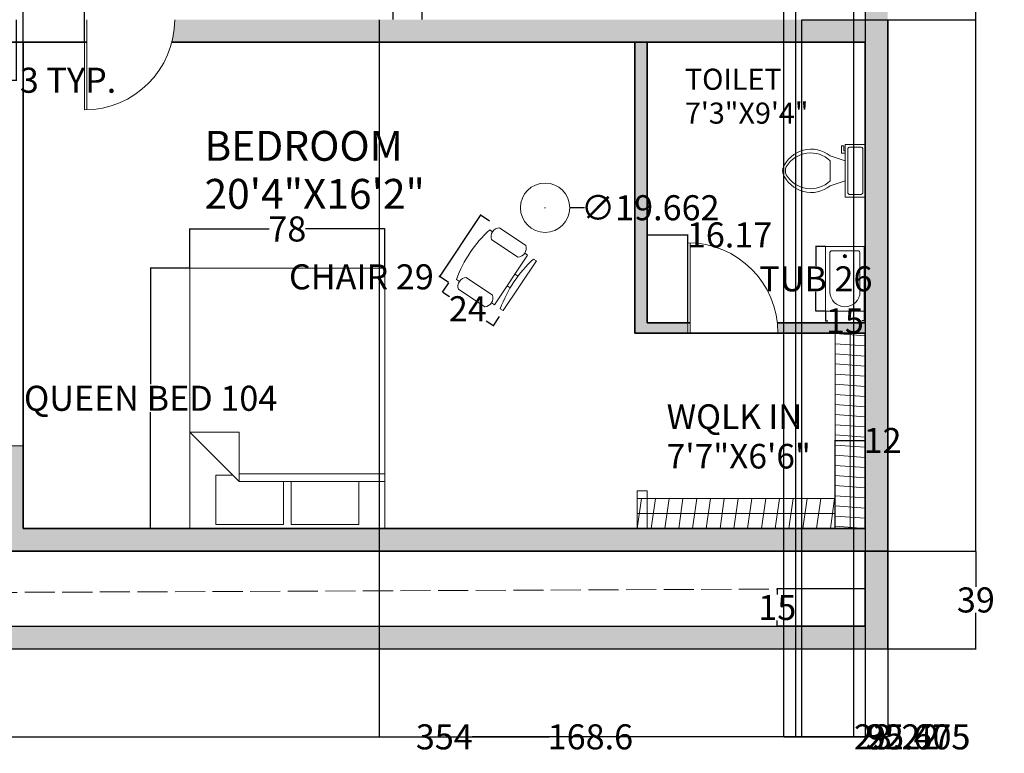
# Model space of a CAD drawing. Units: inches. Extents: x 409 to 1056, y 160 to 945.
# Tile 2 of 6: x 625 to 1018, y 160 to 453. Entities that reach past the tile are written whole.
import ezdxf

# ---------------------------------------------------------------- set-up
doc = ezdxf.new("R2010")
doc.units = ezdxf.units.IN
doc.header["$MEASUREMENT"] = 0
doc.linetypes.add('ACAD_ISO02W100', pattern=[15, 12, -3])
for name, color, linetype, lineweight in [('A-ANNO-DIMS', 2, 'Continuous', 18), ('A-AREA-IDEN', 7, 'Continuous', 18), ('A-DOOR', 3, 'Continuous', 18), ('A-FLOR-CASE', 8, 'Continuous', 20), ('A-FLOR-CASE-PATT', 9, 'Continuous', 13), ('A-FLOR-FIXT', 8, 'Continuous', 18), ('A-FURN', 8, 'Continuous', 18), ('A-GLAZ', 4, 'Continuous', 18), ('A-ROOF-BYND', 8, 'ACAD_ISO02W100', 13), ('A-WALL', 7, 'Continuous', 35), ('A-WALL-PRPT', 7, 'Continuous', 30)]:
    doc.layers.add(name, color=color, linetype=linetype, lineweight=lineweight)
doc.layers.add('A-WALL-PATT', color=251, linetype='Continuous', lineweight=13, true_color=0x636466)
doc.styles.get("Standard").update_dxf_attribs({"font": 'arial.ttf'})
doc.dimstyles.get("Standard").update_dxf_attribs({"dimtxt": 10, "dimasz": 0.18, "dimexe": 0.18, "dimexo": 0.0625, "dimgap": 0.09, "dimtad": 0, "dimtih": 1, "dimtoh": 1, "dimdec": 0, "dimzin": 0, "dimdsep": 46, "dimlunit": 3, "dimtxsty": 'Standard', "dimcen": 0.09, "dimadec": 0, "dimazin": 0, "dimtfac": 1, "dimtdec": 0, "dimtofl": 0, "dimtmove": 0, "dimatfit": 3, "dimfxl": 1, "dimtolj": 1, "dimtzin": 0, "dimarcsym": 0})

# ---------------------------------------------------------------- blocks, each defined once
blk = doc.blocks.new('Bath Tub - 26 x 60 in.')
for p, q in [((8, -18), (10, -18)), ((9, -17), (9, -19))]:
    blk.add_line(p, q)
blk.add_lwpolyline([(0, -36), (0, 0), (60, 0), (60, -36)], close=True)
for points in [[(4, -30), (4, -6)], [(6, -4), (42, -4)], [(42, -32), (6, -32)]]:
    blk.add_lwpolyline(points)
for radius in [1.5, 1]:
    blk.add_circle((9, -18), radius)
for centre, radius, start, end in [((5.75, -5.75), 1.77, 81.8699, 188.1301), ((42, -18), 14, 270, 90), ((5.75, -30.25), 1.77, 171.8699, 278.1301)]:
    blk.add_arc(centre, radius, start, end)
blk = doc.blocks.new('Toilet - top')
for p, q in [((9.5, -6), (9.5, -2)), ((-10, -8.5), (-8, -8.5)), ((-10, -9.5), (-10, -8.5)), ((-7, -9.5), (-10, -9.5)), ((-8, -8.5), (-8, -8)), ((-7, -8), (-7, -9.5)), ((-4, -8), (-6, -14)), ((4, -8), (6, -14)), ((4, -14), (-4, -14))]:
    blk.add_line(p, q)
blk.add_lwpolyline([(10.5, -8), (10.5, 0), (-10.5, 0), (-10.5, -8)], close=True)
for points in [[(-9.5, -2), (-9.5, -6)], [(8.5, -1), (-8.5, -1)], [(-8.5, -7), (8.5, -7)]]:
    blk.add_lwpolyline(points)
for centre, radius, start, end in [((-8.62, -1.88), 0.884, 81.8699, 188.1301), ((8.62, -1.88), 0.884, 351.8699, 98.1301), ((-8.62, -6.12), 0.884, 171.8699, 278.1301), ((8.62, -6.12), 0.884, 261.8699, 8.1301), ((3.52, -21.58), 12.17, 141.4691, 247.9714), ((4.2, -21.82), 11.33, 136.3677, 238.9468), ((-3.52, -21.58), 12.17, 292.0284, 38.5307), ((-4.2, -21.82), 11.33, 301.053, 43.6321), ((0, -27.88), 4, 245.7318, 294.2682), ((0, -29), 4, 254.8605, 285.1395)]:
    blk.add_arc(centre, radius, start, end)
blk = doc.blocks.new('Bed - Queen')
for p, q in [((0, -80.00003), (0, 0)), ((0, 0), (59.99999, 0)), ((59.99999, 0), (59.99999, -80.00003)), ((7.99999, -1.2), (28.79998, -1.2)), ((7.99999, -14.4), (7.99999, -1.2)), ((28.79998, -1.2), (28.79998, -14.4)), ((31.19999, -1.2), (51.99999, -1.2)), ((31.19999, -14.4), (31.19999, -1.2)), ((51.99999, -1.2), (51.99999, -16.4)), ((0, -14.4), (44.8, -14.4)), ((59.99999, -29.6), (44.8, -14.4)), ((44.8, -14.4), (44.8, -29.6)), ((44.8, -16.8), (0, -16.8)), ((51.99999, -16.4), (46.79936, -16.4)), ((44.8, -29.6), (59.99999, -29.6)), ((59.99999, -80.00003), (0, -80.00003))]:
    blk.add_line(p, q)
blk = doc.blocks.new('Chair - Desk')
for p, q in [((-8.5, 0), (-8.5, -1)), ((-8.5, 0), (8.5, 0)), ((8.5, 0), (8.5, -1)), ((-2, -3), (-2, -1.9355)), ((2, -1.9576), (2, -3)), ((-10.5, -5), (-10.5, -14)), ((-8.5, -3), (-8.5, -4)), ((-8.5, -3), (8.5, -3)), ((-6.5, -14), (-6.5, -5)), ((6.5, -5), (6.5, -14)), ((8.5, -3), (8.5, -4)), ((10.5, -14), (10.5, -5)), ((-8.5, -15), (-8.5, -16)), ((8.5, -15), (8.5, -16))]:
    blk.add_line(p, q)
for centre, radius, start, end in [((0, 34.625), 36.625, 256.5803, 283.4197), ((-8.5, -6.5), 2.5, 36.8699, 143.1301), ((8.5, -6.5), 2.5, 36.8699, 143.1301), ((-8.5, -12.5), 2.5, 216.8699, 323.1301), ((8.5, -12.5), 2.5, 216.8699, 323.1301), ((0, 19.625), 36.625, 256.5803, 283.4197)]:
    blk.add_arc(centre, radius, start, end)
blk = doc.blocks.new('DOOR-SWING-36IN')
for p, q in [((35, 36), (35, 0)), ((36, 36), (36, 0))]:
    blk.add_line(p, q)
blk.add_arc((36, 36), 36, 180, 270)
blk = doc.blocks.new('*D14')
at = {"layer": 'A-ANNO-DIMS', "color": 0, "lineweight": -2, "transparency": 16777216}
for p, q in [((620.85, 452.68), (620.85, 428.41)), ((623.85, 452.68), (623.85, 428.41)), ((621.03, 428.59), (623.67, 428.59)), ((623.85, 428.59), (624.03, 428.59))]:
    blk.add_line(p, q, dxfattribs=at)
at = {"layer": 'A-ANNO-DIMS', "color": 0, "transparency": 16777216}
for points in [[(621.03, 428.62), (621.03, 428.56), (620.85, 428.59)], [(623.67, 428.62), (623.67, 428.56), (623.85, 428.59)]]:
    blk.add_solid(points, dxfattribs=at)
at = {"layer": 'Defpoints', "color": 0, "transparency": 16777216}
for p in [(620.85, 452.74), (623.85, 452.74), (623.85, 428.59)]:
    blk.add_point(p, dxfattribs=at)
at = {"layer": 'A-ANNO-DIMS', "color": 0, "transparency": 16777216, "insert": (644.57, 428.59), "char_height": 10, "attachment_point": 5}
blk.add_mtext('\\A1;3 TYP.', dxfattribs=at)
blk = doc.blocks.new('*D15')
at = {"layer": 'A-ANNO-DIMS', "color": 0, "lineweight": -2, "transparency": 16777216}
for p, q in [((693.07, 353.66), (677.36, 353.66)), ((677.54, 353.48), (677.54, 307.27)), ((677.54, 249.92), (677.54, 296.13)), ((693.07, 249.74), (677.36, 249.74))]:
    blk.add_line(p, q, dxfattribs=at)
at = {"layer": 'A-ANNO-DIMS', "color": 0, "transparency": 16777216}
for points in [[(677.51, 353.48), (677.57, 353.48), (677.54, 353.66)], [(677.51, 249.92), (677.57, 249.92), (677.54, 249.74)]]:
    blk.add_solid(points, dxfattribs=at)
at = {"layer": 'Defpoints', "color": 0, "transparency": 16777216}
for p in [(693.13, 353.66), (677.54, 249.74), (693.13, 249.74)]:
    blk.add_point(p, dxfattribs=at)
at = {"layer": 'A-ANNO-DIMS', "color": 0, "transparency": 16777216, "insert": (677.54, 301.7), "char_height": 10, "attachment_point": 5}
blk.add_mtext('\\A1;QUEEN BED 104', dxfattribs=at)
blk = doc.blocks.new('*D16')
at = {"layer": 'A-ANNO-DIMS', "color": 0, "lineweight": -2, "transparency": 16777216}
for p, q in [((693.13, 353.72), (693.13, 369.43)), ((771.07, 353.72), (771.07, 369.43)), ((693.31, 369.25), (724.88, 369.25)), ((770.89, 369.25), (739.32, 369.25))]:
    blk.add_line(p, q, dxfattribs=at)
at = {"layer": 'A-ANNO-DIMS', "color": 0, "transparency": 16777216}
for points in [[(693.31, 369.28), (693.31, 369.22), (693.13, 369.25)], [(770.89, 369.28), (770.89, 369.22), (771.07, 369.25)]]:
    blk.add_solid(points, dxfattribs=at)
at = {"layer": 'Defpoints', "color": 0, "transparency": 16777216}
for p in [(693.13, 369.25), (693.13, 353.66), (771.07, 353.66)]:
    blk.add_point(p, dxfattribs=at)
at = {"layer": 'A-ANNO-DIMS', "color": 0, "transparency": 16777216, "insert": (732.1, 369.25), "char_height": 10, "attachment_point": 5}
blk.add_mtext('\\A1;78', dxfattribs=at)
blk = doc.blocks.new('*D17')
at = {"layer": 'A-ANNO-DIMS', "color": 0, "lineweight": -2, "transparency": 16777216}
for p, q in [((809.08, 374.62), (792.92, 350.44)), ((812.8, 372.35), (809.03, 374.87)), ((792.72, 350.15), (792.54, 350.15)), ((796.44, 347.88), (792.67, 350.4)), ((792.82, 350.3), (792.72, 350.15))]:
    blk.add_line(p, q, dxfattribs=at)
at = {"layer": 'A-ANNO-DIMS', "color": 0, "transparency": 16777216}
for points in [[(809.06, 374.64), (809.11, 374.6), (809.18, 374.77)], [(792.9, 350.46), (792.95, 350.43), (792.82, 350.3)]]:
    blk.add_solid(points, dxfattribs=at)
at = {"layer": 'Defpoints', "color": 0, "transparency": 16777216}
for p in [(812.86, 372.31), (792.82, 350.3), (796.49, 347.84)]:
    blk.add_point(p, dxfattribs=at)
at = {"layer": 'A-ANNO-DIMS', "color": 0, "transparency": 16777216, "insert": (761.66, 350.15), "char_height": 10, "attachment_point": 5}
blk.add_mtext('\\A1;CHAIR 29', dxfattribs=at)
blk = doc.blocks.new('*D18')
at = {"layer": 'A-ANNO-DIMS', "color": 0, "lineweight": -2, "transparency": 16777216}
for p, q in [((796.46, 347.79), (793.94, 344.02)), ((794.19, 344.07), (796.82, 342.31)), ((816.66, 334.28), (814.14, 330.51)), ((814.09, 330.76), (811.45, 332.52))]:
    blk.add_line(p, q, dxfattribs=at)
at = {"layer": 'A-ANNO-DIMS', "color": 0, "transparency": 16777216}
for points in [[(794.2, 344.09), (794.17, 344.04), (794.04, 344.17)], [(814.1, 330.79), (814.07, 330.74), (814.24, 330.66)]]:
    blk.add_solid(points, dxfattribs=at)
at = {"layer": 'Defpoints', "color": 0, "transparency": 16777216}
for p in [(796.49, 347.84), (816.69, 334.33), (814.24, 330.66)]:
    blk.add_point(p, dxfattribs=at)
at = {"layer": 'A-ANNO-DIMS', "color": 0, "transparency": 16777216, "insert": (804.14, 337.42), "char_height": 10, "attachment_point": 5}
blk.add_mtext('\\A1;24', dxfattribs=at)
blk = doc.blocks.new('*D29')
at = {"layer": 'A-ANNO-DIMS', "color": 0, "lineweight": -2, "transparency": 16777216}
for p, q in [((946.82, 362.24), (942.84, 362.24)), ((943.02, 362.06), (943.02, 354.55)), ((943.02, 336.65), (943.02, 344.16)), ((946.82, 336.47), (942.84, 336.47))]:
    blk.add_line(p, q, dxfattribs=at)
at = {"layer": 'A-ANNO-DIMS', "color": 0, "transparency": 16777216}
for points in [[(942.99, 362.06), (943.05, 362.06), (943.02, 362.24)], [(942.99, 336.65), (943.05, 336.65), (943.02, 336.47)]]:
    blk.add_solid(points, dxfattribs=at)
at = {"layer": 'Defpoints', "color": 0, "transparency": 16777216}
for p in [(946.88, 362.24), (943.02, 336.47), (946.88, 336.47)]:
    blk.add_point(p, dxfattribs=at)
at = {"layer": 'A-ANNO-DIMS', "color": 0, "transparency": 16777216, "insert": (943.02, 349.36), "char_height": 10, "attachment_point": 5}
blk.add_mtext('\\A1;TUB 26', dxfattribs=at)
blk = doc.blocks.new('*D30')
at = {"layer": 'A-ANNO-DIMS', "color": 0, "lineweight": -2, "transparency": 16777216}
for p, q in [((946.88, 336.41), (946.88, 332.43)), ((962.34, 336.41), (962.34, 332.43)), ((947.06, 332.61), (947.79, 332.61)), ((962.16, 332.61), (961.43, 332.61))]:
    blk.add_line(p, q, dxfattribs=at)
at = {"layer": 'A-ANNO-DIMS', "color": 0, "transparency": 16777216}
for points in [[(947.06, 332.64), (947.06, 332.58), (946.88, 332.61)], [(962.16, 332.64), (962.16, 332.58), (962.34, 332.61)]]:
    blk.add_solid(points, dxfattribs=at)
at = {"layer": 'Defpoints', "color": 0, "transparency": 16777216}
for p in [(946.88, 336.47), (962.34, 336.47), (962.34, 332.61)]:
    blk.add_point(p, dxfattribs=at)
at = {"layer": 'A-ANNO-DIMS', "color": 0, "transparency": 16777216, "insert": (954.61, 332.61), "char_height": 10, "attachment_point": 5}
blk.add_mtext('\\A1;15', dxfattribs=at)
blk = doc.blocks.new('*D37')
at = {"layer": 'A-ANNO-DIMS', "color": 0, "lineweight": -2, "transparency": 16777216}
for p, q in [((617.74, 240.68), (617.74, 166.44)), ((971.74, 240.68), (971.74, 166.44)), ((617.92, 166.62), (783.63, 166.62)), ((971.56, 166.62), (805.85, 166.62))]:
    blk.add_line(p, q, dxfattribs=at)
at = {"layer": 'A-ANNO-DIMS', "color": 0, "transparency": 16777216}
for points in [[(617.92, 166.65), (617.92, 166.59), (617.74, 166.62)], [(971.56, 166.65), (971.56, 166.59), (971.74, 166.62)]]:
    blk.add_solid(points, dxfattribs=at)
at = {"layer": 'Defpoints', "color": 0, "transparency": 16777216}
for p in [(617.74, 240.74), (971.74, 240.74), (971.74, 166.62)]:
    blk.add_point(p, dxfattribs=at)
at = {"layer": 'A-ANNO-DIMS', "color": 0, "transparency": 16777216, "insert": (794.74, 166.62), "char_height": 10, "attachment_point": 5}
blk.add_mtext('\\A1;354', dxfattribs=at)
blk = doc.blocks.new('*D38')
at = {"layer": 'A-ANNO-DIMS', "color": 0, "lineweight": -2, "transparency": 16777216}
for p, q in [((971.8, 810.74), (1007.05, 810.74)), ((1006.87, 810.56), (1006.87, 530.94)), ((1006.87, 240.92), (1006.87, 520.55)), ((971.8, 240.74), (1007.05, 240.74))]:
    blk.add_line(p, q, dxfattribs=at)
at = {"layer": 'A-ANNO-DIMS', "color": 0, "transparency": 16777216}
for points in [[(1006.84, 810.56), (1006.9, 810.56), (1006.87, 810.74)], [(1006.84, 240.92), (1006.9, 240.92), (1006.87, 240.74)]]:
    blk.add_solid(points, dxfattribs=at)
at = {"layer": 'Defpoints', "color": 0, "transparency": 16777216}
for p in [(971.74, 810.74), (1006.87, 810.74), (971.74, 240.74)]:
    blk.add_point(p, dxfattribs=at)
at = {"layer": 'A-ANNO-DIMS', "color": 0, "transparency": 16777216, "insert": (1006.87, 525.74), "char_height": 10, "attachment_point": 5}
blk.add_mtext('\\A1;570', dxfattribs=at)
blk = doc.blocks.new('*D39')
at = {"layer": 'A-ANNO-DIMS', "color": 0, "lineweight": -2, "transparency": 16777216}
for p, q in [((971.8, 240.74), (1007.05, 240.74)), ((1006.87, 240.56), (1006.87, 226.44)), ((1006.87, 201.92), (1006.87, 216.04)), ((971.8, 201.74), (1007.05, 201.74))]:
    blk.add_line(p, q, dxfattribs=at)
at = {"layer": 'A-ANNO-DIMS', "color": 0, "transparency": 16777216}
for points in [[(1006.84, 240.56), (1006.9, 240.56), (1006.87, 240.74)], [(1006.84, 201.92), (1006.9, 201.92), (1006.87, 201.74)]]:
    blk.add_solid(points, dxfattribs=at)
at = {"layer": 'Defpoints', "color": 0, "transparency": 16777216}
for p in [(971.74, 240.74), (1006.87, 240.74), (971.74, 201.74)]:
    blk.add_point(p, dxfattribs=at)
at = {"layer": 'A-ANNO-DIMS', "color": 0, "transparency": 16777216, "insert": (1006.87, 221.24), "char_height": 10, "attachment_point": 5}
blk.add_mtext('\\A1;39', dxfattribs=at)
blk = doc.blocks.new('*D40')
at = {"layer": 'A-ANNO-DIMS', "color": 0, "lineweight": -2, "transparency": 16777216}
for p, q in [((930.07, 622.68), (930.07, 166.44)), ((962.74, 622.68), (962.74, 166.44)), ((930.25, 166.62), (962.56, 166.62)), ((962.74, 166.62), (962.92, 166.62))]:
    blk.add_line(p, q, dxfattribs=at)
at = {"layer": 'A-ANNO-DIMS', "color": 0, "transparency": 16777216}
for points in [[(930.25, 166.65), (930.25, 166.59), (930.07, 166.62)], [(962.56, 166.65), (962.56, 166.59), (962.74, 166.62)]]:
    blk.add_solid(points, dxfattribs=at)
at = {"layer": 'Defpoints', "color": 0, "transparency": 16777216}
for p in [(930.07, 622.74), (962.74, 622.74), (962.74, 166.62)]:
    blk.add_point(p, dxfattribs=at)
at = {"layer": 'A-ANNO-DIMS', "color": 0, "transparency": 16777216, "insert": (983.8, 166.62), "char_height": 10, "attachment_point": 5}
blk.add_mtext('\\A1;32.675', dxfattribs=at)
blk = doc.blocks.new('*D41')
at = {"layer": 'A-ANNO-DIMS', "color": 0, "lineweight": -2, "transparency": 16777216}
for p, q in [((934.87, 626.08), (934.87, 166.44)), ((958.09, 626.08), (958.09, 166.44)), ((935.05, 166.62), (957.91, 166.62)), ((958.09, 166.62), (958.27, 166.62))]:
    blk.add_line(p, q, dxfattribs=at)
at = {"layer": 'A-ANNO-DIMS', "color": 0, "transparency": 16777216}
for points in [[(935.05, 166.65), (935.05, 166.59), (934.87, 166.62)], [(957.91, 166.65), (957.91, 166.59), (958.09, 166.62)]]:
    blk.add_solid(points, dxfattribs=at)
at = {"layer": 'Defpoints', "color": 0, "transparency": 16777216}
for p in [(934.87, 626.14), (958.09, 626.14), (958.09, 166.62)]:
    blk.add_point(p, dxfattribs=at)
at = {"layer": 'A-ANNO-DIMS', "color": 0, "transparency": 16777216, "insert": (975.27, 166.62), "char_height": 10, "attachment_point": 5}
blk.add_mtext('\\A1;23.22', dxfattribs=at)
blk = doc.blocks.new('*D45')
at = {"layer": 'A-ANNO-DIMS', "color": 0, "lineweight": -2, "transparency": 16777216}
for p, q in [((962.74, 452.68), (962.74, 166.44)), ((971.74, 443.68), (971.74, 166.44)), ((962.92, 166.62), (963.86, 166.62)), ((971.56, 166.62), (970.62, 166.62))]:
    blk.add_line(p, q, dxfattribs=at)
at = {"layer": 'A-ANNO-DIMS', "color": 0, "transparency": 16777216}
for points in [[(962.92, 166.65), (962.92, 166.59), (962.74, 166.62)], [(971.56, 166.65), (971.56, 166.59), (971.74, 166.62)]]:
    blk.add_solid(points, dxfattribs=at)
at = {"layer": 'Defpoints', "color": 0, "transparency": 16777216}
for p in [(962.74, 452.74), (971.74, 443.74), (971.74, 166.62)]:
    blk.add_point(p, dxfattribs=at)
at = {"layer": 'A-ANNO-DIMS', "color": 0, "transparency": 16777216, "insert": (967.24, 166.62), "char_height": 10, "attachment_point": 5}
blk.add_mtext('\\A1;9', dxfattribs=at)
blk = doc.blocks.new('*D48')
at = {"layer": 'A-ANNO-DIMS', "color": 0, "lineweight": -2, "transparency": 16777216}
for p, q in [((768.74, 452.68), (768.74, 166.44)), ((937.34, 452.68), (937.34, 166.44)), ((768.92, 166.62), (836.55, 166.62)), ((937.16, 166.62), (869.53, 166.62))]:
    blk.add_line(p, q, dxfattribs=at)
at = {"layer": 'A-ANNO-DIMS', "color": 0, "transparency": 16777216}
for points in [[(768.92, 166.65), (768.92, 166.59), (768.74, 166.62)], [(937.16, 166.65), (937.16, 166.59), (937.34, 166.62)]]:
    blk.add_solid(points, dxfattribs=at)
at = {"layer": 'Defpoints', "color": 0, "transparency": 16777216}
for p in [(768.74, 452.74), (937.34, 452.74), (937.34, 166.62)]:
    blk.add_point(p, dxfattribs=at)
at = {"layer": 'A-ANNO-DIMS', "color": 0, "transparency": 16777216, "insert": (853.04, 166.62), "char_height": 10, "attachment_point": 5}
blk.add_mtext('\\A1;168.6', dxfattribs=at)
blk = doc.blocks.new('*D49')
at = {"layer": 'A-ANNO-DIMS', "color": 0, "lineweight": -2, "transparency": 16777216}
for p, q in [((937.4, 539.74), (1007.05, 539.74)), ((1006.87, 539.56), (1006.87, 501.44)), ((1006.87, 452.92), (1006.87, 491.05)), ((937.4, 452.74), (1007.05, 452.74))]:
    blk.add_line(p, q, dxfattribs=at)
at = {"layer": 'A-ANNO-DIMS', "color": 0, "transparency": 16777216}
for points in [[(1006.84, 539.56), (1006.9, 539.56), (1006.87, 539.74)], [(1006.84, 452.92), (1006.9, 452.92), (1006.87, 452.74)]]:
    blk.add_solid(points, dxfattribs=at)
at = {"layer": 'Defpoints', "color": 0, "transparency": 16777216}
for p in [(937.34, 539.74), (1006.87, 539.74), (937.34, 452.74)]:
    blk.add_point(p, dxfattribs=at)
at = {"layer": 'A-ANNO-DIMS', "color": 0, "transparency": 16777216, "insert": (1006.87, 496.24), "char_height": 10, "attachment_point": 5}
blk.add_mtext('\\A1;87', dxfattribs=at)
blk = doc.blocks.new('*D50')
at = {"layer": 'A-ANNO-DIMS', "color": 0, "lineweight": -2, "transparency": 16777216}
for p, q in [((937.34, 452.68), (937.34, 166.44)), ((962.74, 452.68), (962.74, 166.44)), ((937.52, 166.62), (962.56, 166.62)), ((962.74, 166.62), (962.92, 166.62))]:
    blk.add_line(p, q, dxfattribs=at)
at = {"layer": 'A-ANNO-DIMS', "color": 0, "transparency": 16777216}
for points in [[(937.52, 166.65), (937.52, 166.59), (937.34, 166.62)], [(962.56, 166.65), (962.56, 166.59), (962.74, 166.62)]]:
    blk.add_solid(points, dxfattribs=at)
at = {"layer": 'Defpoints', "color": 0, "transparency": 16777216}
for p in [(937.34, 452.74), (962.74, 452.74), (962.74, 166.62)]:
    blk.add_point(p, dxfattribs=at)
at = {"layer": 'A-ANNO-DIMS', "color": 0, "transparency": 16777216, "insert": (983.89, 166.62), "char_height": 10, "attachment_point": 5}
blk.add_mtext('\\A1;25.405', dxfattribs=at)
blk = doc.blocks.new('*D53')
at = {"layer": 'A-ANNO-DIMS', "color": 0, "lineweight": -2, "transparency": 16777216}
for p, q in [((774.31, 452.81), (774.31, 939.05)), ((774.49, 938.87), (785.78, 938.87)), ((785.96, 452.81), (785.96, 939.05)), ((785.96, 938.87), (786.14, 938.87))]:
    blk.add_line(p, q, dxfattribs=at)
at = {"layer": 'A-ANNO-DIMS', "color": 0, "transparency": 16777216}
for points in [[(774.49, 938.9), (774.49, 938.84), (774.31, 938.87)], [(785.78, 938.9), (785.78, 938.84), (785.96, 938.87)]]:
    blk.add_solid(points, dxfattribs=at)
at = {"layer": 'Defpoints', "color": 0, "transparency": 16777216}
for p in [(785.96, 938.87), (774.31, 452.74), (785.96, 452.74)]:
    blk.add_point(p, dxfattribs=at)
at = {"layer": 'A-ANNO-DIMS', "color": 0, "transparency": 16777216, "insert": (806.55, 938.87), "char_height": 10, "attachment_point": 5}
blk.add_mtext('\\A1;11.645', dxfattribs=at)
blk = doc.blocks.new('*D55')
at = {"layer": 'A-ANNO-DIMS', "color": 0, "lineweight": -2, "transparency": 16777216}
for p, q in [((626.74, 443.81), (626.74, 479.05)), ((626.92, 478.87), (650.97, 478.87)), ((651.15, 443.81), (651.15, 479.05)), ((651.15, 478.87), (651.33, 478.87))]:
    blk.add_line(p, q, dxfattribs=at)
at = {"layer": 'A-ANNO-DIMS', "color": 0, "transparency": 16777216}
for points in [[(626.92, 478.9), (626.92, 478.84), (626.74, 478.87)], [(650.97, 478.9), (650.97, 478.84), (651.15, 478.87)]]:
    blk.add_solid(points, dxfattribs=at)
at = {"layer": 'Defpoints', "color": 0, "transparency": 16777216}
for p in [(651.15, 478.87), (626.74, 443.74), (651.15, 443.74)]:
    blk.add_point(p, dxfattribs=at)
at = {"layer": 'A-ANNO-DIMS', "color": 0, "transparency": 16777216, "insert": (667.41, 478.87), "char_height": 10, "attachment_point": 5}
blk.add_mtext('\\A1;24.41', dxfattribs=at)
blk = doc.blocks.new('*D56')
at = {"layer": 'A-ANNO-DIMS', "color": 0, "lineweight": -2, "transparency": 16777216}
for p, q in [((875.74, 331.81), (875.74, 367.05)), ((875.92, 366.87), (891.73, 366.87)), ((891.91, 331.81), (891.91, 367.05)), ((891.91, 366.87), (892.09, 366.87))]:
    blk.add_line(p, q, dxfattribs=at)
at = {"layer": 'A-ANNO-DIMS', "color": 0, "transparency": 16777216}
for points in [[(875.92, 366.9), (875.92, 366.84), (875.74, 366.87)], [(891.73, 366.9), (891.73, 366.84), (891.91, 366.87)]]:
    blk.add_solid(points, dxfattribs=at)
at = {"layer": 'Defpoints', "color": 0, "transparency": 16777216}
for p in [(891.91, 366.87), (875.74, 331.74), (891.91, 331.74)]:
    blk.add_point(p, dxfattribs=at)
at = {"layer": 'A-ANNO-DIMS', "color": 0, "transparency": 16777216, "insert": (908.58, 366.87), "char_height": 10, "attachment_point": 5}
blk.add_mtext('\\A1;16.17', dxfattribs=at)
blk = doc.blocks.new('*D62')
at = {"layer": 'A-ANNO-DIMS', "color": 0, "lineweight": -2, "transparency": 16777216}
for p, q in [((962.68, 225.74), (927.44, 225.74)), ((927.62, 225.56), (927.62, 223.44)), ((927.62, 210.92), (927.62, 213.05)), ((962.68, 210.74), (927.44, 210.74))]:
    blk.add_line(p, q, dxfattribs=at)
at = {"layer": 'A-ANNO-DIMS', "color": 0, "transparency": 16777216}
for points in [[(927.59, 225.56), (927.65, 225.56), (927.62, 225.74)], [(927.59, 210.92), (927.65, 210.92), (927.62, 210.74)]]:
    blk.add_solid(points, dxfattribs=at)
at = {"layer": 'Defpoints', "color": 0, "transparency": 16777216}
for p in [(927.62, 225.74), (962.74, 225.74), (962.74, 210.74)]:
    blk.add_point(p, dxfattribs=at)
at = {"layer": 'A-ANNO-DIMS', "color": 0, "transparency": 16777216, "insert": (927.62, 218.24), "char_height": 10, "attachment_point": 5}
blk.add_mtext('\\A1;15', dxfattribs=at)
blk = doc.blocks.new('*D63')
at = {"layer": 'A-ANNO-DIMS', "color": 0, "lineweight": -2, "transparency": 16777216}
for p, q in [((950.74, 249.81), (950.74, 285.05)), ((950.92, 284.87), (962.56, 284.87)), ((962.74, 249.81), (962.74, 285.05)), ((962.74, 284.87), (962.92, 284.87))]:
    blk.add_line(p, q, dxfattribs=at)
at = {"layer": 'A-ANNO-DIMS', "color": 0, "transparency": 16777216}
for points in [[(950.92, 284.9), (950.92, 284.84), (950.74, 284.87)], [(962.56, 284.9), (962.56, 284.84), (962.74, 284.87)]]:
    blk.add_solid(points, dxfattribs=at)
at = {"layer": 'Defpoints', "color": 0, "transparency": 16777216}
for p in [(962.74, 284.87), (950.74, 249.74), (962.74, 249.74)]:
    blk.add_point(p, dxfattribs=at)
at = {"layer": 'A-ANNO-DIMS', "color": 0, "transparency": 16777216, "insert": (969.65, 284.87), "char_height": 10, "attachment_point": 5}
blk.add_mtext('\\A1;12', dxfattribs=at)
blk = doc.blocks.new('*D66')
at = {"layer": 'A-ANNO-DIMS', "color": 0, "lineweight": -2, "transparency": 16777216}
for p, q in [((834.88, 377.72), (835.06, 377.72)), ((834.97, 377.63), (834.97, 377.81)), ((850.69, 377.72), (844.98, 377.72))]:
    blk.add_line(p, q, dxfattribs=at)
at = {"layer": 'A-ANNO-DIMS', "color": 0, "transparency": 16777216}
blk.add_solid([(844.98, 377.75), (844.98, 377.69), (844.8, 377.72)], dxfattribs=at)
at = {"layer": 'Defpoints', "color": 0, "transparency": 16777216}
for p in [(825.13, 377.72), (844.8, 377.72)]:
    blk.add_point(p, dxfattribs=at)
at = {"layer": 'A-ANNO-DIMS', "color": 0, "transparency": 16777216, "insert": (876.93, 377.72), "char_height": 10, "attachment_point": 5}
blk.add_mtext('\\A1;∅19.662', dxfattribs=at)

msp = doc.modelspace()

# ---------------------------------------------------------------- hatches: boundary and pattern name
at = {"layer": 'A-FLOR-CASE-PATT'}
h = msp.add_hatch(dxfattribs=at)
h.set_pattern_fill('ANSI31', color=256, scale=32.27711, angle=130.8546, style=0)
h.paths.add_polyline_path([(950.7418, 249.7439), (962.7418, 249.7439), (962.7418, 327.7439), (950.7418, 327.7439)])
h = msp.add_hatch(dxfattribs=at)
h.set_pattern_fill('ANSI31', color=256, scale=43.5863, angle=36.9402, style=0)
h.paths.add_polyline_path([(871.7418, 249.7439), (950.7418, 249.7439), (950.7418, 261.7439), (871.7418, 261.7439)])
at = {"layer": 'A-WALL-PATT'}
h = msp.add_hatch(color=256, dxfattribs=at)
h.dxf.hatch_style = 1
h.paths.add_polyline_path([(730.4481, 698.1956), (696.9841, 709.3369, 1), (696.9841, 678.8752)], flags=17)
h.paths.add_polyline_path([(803.8768, 698.1956), (770.4128, 709.3369, 1), (770.4128, 678.8752)], flags=17)
h.paths.add_polyline_path([(464.7418, 894.7439), (466.7418, 894.7439), (962.7418, 894.7439), (962.7418, 810.7439), (971.7418, 810.7439), (971.7418, 903.7439), (455.7418, 903.7439), (455.7418, 201.7439), (971.7418, 201.7439), (971.7418, 240.7439), (962.7418, 240.7439), (962.7418, 210.7439), (464.7418, 210.7439)])
h = msp.add_hatch(color=256, dxfattribs=at)
h.dxf.hatch_style = 1
h.paths.add_polyline_path([(626.7418, 801.7439), (870.7418, 801.7439), (870.7418, 710.7439), (870.7418, 683.9043), (875.7418, 683.9043), (875.7418, 707.7439), (962.7418, 707.7439), (962.7418, 710.7439), (875.7418, 710.7439), (875.7418, 722.7439), (875.7418, 801.7439), (885.6955, 801.7439, -0.06325422), (884.5523, 810.7439), (617.7418, 810.7439), (617.7418, 732.9297), (626.7418, 732.9297)])
h.paths.add_polyline_path([(962.7418, 810.7439), (920.5523, 810.7439), (920.5523, 801.7439), (962.7418, 801.7439)], flags=17)
h.paths.add_polyline_path([(971.7418, 810.7439), (962.7418, 810.7439), (962.7418, 801.7439), (962.7418, 707.7439), (962.7418, 622.7439), (962.7418, 613.7439), (962.7418, 548.7439), (856.7418, 548.7439), (847.7418, 548.7439), (776.7418, 548.7439), (776.7418, 569.8172), (768.7418, 569.8172), (768.7418, 539.7439), (847.7418, 539.7439), (971.7418, 539.7439), (971.7418, 613.7439), (971.7418, 707.7439)])
h.paths.add_polyline_path([(883.2418, 622.7439), (875.7418, 622.7439), (684.4993, 622.7439, -0.06325422), (685.6424, 613.7439), (870.7418, 613.7439), (875.7418, 613.7439), (884.3849, 613.7439, -0.06325422)])
h.paths.add_polyline_path([(649.6424, 622.7439), (626.7418, 622.7439), (626.7418, 613.7439), (649.6424, 613.7439)])
h.paths.add_polyline_path([(626.7418, 652.3165), (617.7418, 652.3165), (617.7418, 613.7439), (626.7418, 613.7439), (626.7418, 622.7439)])
h.paths.add_polyline_path([(776.7418, 613.7439), (768.7418, 613.7439), (768.7418, 590.4138), (776.7418, 590.4138)], flags=17)
h.paths.add_polyline_path([(856.7418, 613.7439), (847.7418, 613.7439), (847.7418, 548.7439), (856.7418, 548.7439)], flags=17)
h.paths.add_polyline_path([(962.7418, 622.7439), (919.2418, 622.7439), (919.2418, 613.7439), (962.7418, 613.7439)], flags=17)
h.paths.add_polyline_path([(971.7418, 539.7439), (962.7418, 539.7439), (962.7418, 452.7439), (687.1506, 452.7439, -0.06325422), (686.0074, 443.7439), (962.7418, 443.7439), (962.7418, 331.7439), (927.6873, 331.7439, -0.02784244), (927.9102, 327.7439), (962.7418, 327.7439), (962.7418, 249.7439), (871.7418, 249.7439), (870.7418, 249.7439), (626.7418, 249.7439), (626.7418, 282.7439), (617.7418, 282.7439), (617.7418, 240.7439), (870.7418, 240.7439), (871.7418, 240.7439), (971.7418, 240.7439), (971.7418, 249.7439), (971.7418, 327.7439), (971.7418, 331.7439), (971.7418, 443.7439), (971.7418, 452.7439)])
h.paths.add_polyline_path([(875.7418, 443.7439), (870.7418, 443.7439), (870.7418, 327.7439), (871.7418, 327.7439), (891.9102, 327.7439), (891.9102, 331.7439), (875.7418, 331.7439)], flags=17)

# ---------------------------------------------------------------- linework, layer by layer
at = {"layer": 'A-DOOR'}
for p, q in [((651.1506, 452.7439), (651.1506, 443.7439)), ((891.9102, 327.7439), (891.9102, 331.7439)), ((891.9102, 327.7439), (927.9102, 327.7439))]:
    msp.add_line(p, q, dxfattribs=at)
at = {"layer": 'A-FLOR-CASE'}
for p, q in [((962.7418, 327.7439), (950.7418, 327.7439)), ((950.7418, 327.7439), (950.7418, 249.7439)), ((956.7418, 327.7439), (956.7418, 249.7439)), ((871.7418, 261.7439), (871.7418, 264.8034)), ((871.7418, 264.8034), (875.7418, 264.8034)), ((875.7418, 249.7439), (875.7418, 264.8034)), ((871.7418, 249.7439), (871.7418, 261.7439)), ((871.7418, 261.7439), (944.0879, 261.7439)), ((950.7418, 261.7439), (938.757, 261.7439)), ((871.7418, 255.7439), (950.7418, 255.7439))]:
    msp.add_line(p, q, dxfattribs=at)
at = {"layer": 'A-FURN'}
msp.add_circle((834.9651, 377.7213), 9.8311, dxfattribs=at)
at = {"layer": 'A-GLAZ'}
msp.add_line((617.7418, 282.7439), (626.7418, 282.7439), dxfattribs=at)
at = {"layer": 'A-ROOF-BYND'}
msp.add_line((537.2978, 223.8898), (962.7418, 225.7439), dxfattribs=at)
at = {"layer": 'A-WALL'}
for p, q in [((971.7418, 443.7439), (971.7418, 452.7439)), ((617.7418, 443.7439), (652.1506, 443.7439)), ((626.7418, 443.7439), (626.7418, 249.7439)), ((686.0074, 443.7439), (962.7418, 443.7439)), ((870.7418, 327.7439), (870.7418, 443.7439)), ((875.7418, 331.7439), (875.7418, 443.7439)), ((962.7418, 331.7439), (962.7418, 443.7439)), ((971.7418, 331.7439), (971.7418, 443.7439)), ((892.9102, 331.7439), (875.7418, 331.7439)), ((962.7418, 331.7439), (927.6873, 331.7439)), ((971.7418, 327.7439), (971.7418, 331.7439)), ((871.7418, 327.7439), (870.7418, 327.7439)), ((962.7418, 327.7439), (871.7418, 327.7439)), ((962.7418, 249.7439), (962.7418, 327.7439)), ((971.7418, 249.7439), (971.7418, 327.7439)), ((626.7418, 249.7439), (870.7418, 249.7439)), ((870.7418, 249.7439), (871.7418, 249.7439)), ((871.7418, 249.7439), (962.7418, 249.7439)), ((971.7418, 249.7439), (971.7418, 240.7439)), ((617.7418, 240.7439), (870.7418, 240.7439)), ((871.7418, 240.7439), (870.7418, 240.7439)), ((871.7418, 240.7439), (971.7418, 240.7439))]:
    msp.add_line(p, q, dxfattribs=at)
at = {"layer": 'A-WALL-PRPT'}
for p, q in [((962.7418, 210.7439), (962.7418, 240.7439)), ((971.7418, 201.7439), (971.7418, 240.7439)), ((464.7418, 210.7439), (962.7418, 210.7439)), ((455.7418, 201.7439), (971.7418, 201.7439))]:
    msp.add_line(p, q, dxfattribs=at)

# ---------------------------------------------------------------- block references
at = {"layer": 'A-DOOR', "extrusion": (0, 0, -1), "zscale": -1}
msp.add_blockref('DOOR-SWING-36IN', (-687.1509, 416.744), dxfattribs=at)
at = {"layer": 'A-DOOR', "rotation": 180}
msp.add_blockref('DOOR-SWING-36IN', (927.9106, 363.7438), dxfattribs=at)
at = {"layer": 'A-FLOR-FIXT', "rotation": 270}
msp.add_blockref('Toilet - top', (962.7418, 392.4535), dxfattribs=at)
at = {"layer": 'A-FLOR-FIXT', "xscale": 0.4294042930034013, "yscale": 0.4294042930034013, "zscale": 0.4294042930034013, "rotation": 269.9999999999994}
msp.add_blockref('Bath Tub - 26 x 60 in.', (962.3432, 362.2375), dxfattribs=at)
at = {"layer": 'A-FURN'}
for name, p, xscale, yscale, zscale, rotation in [('Chair - Desk', (824.873, 346.5702), 1.401898914076893, 1.401898914076893, 1.401898914076893, 236.2310783252297), ('Bed - Queen', (771.0682, 249.7439), 1.298961397598499, 1.298961397598499, 1.298961397598499, 180)]:
    msp.add_blockref(name, p, dxfattribs=dict(at, xscale=xscale, yscale=yscale, zscale=zscale, rotation=rotation))

# ---------------------------------------------------------------- texts
at = {"layer": 'A-AREA-IDEN'}
for s, height, p in [('TOILET ', 8.41266, (890.7574, 424.7793)), ('7\'3"X9\'4"', 8.41266, (890.7574, 411.2651)), ('BEDROOM ', 11.92421, (699.0308, 396.4502)), ('20\'4"X16\'2"', 11.924212, (699.0308, 377.295)), ('WQLK IN ', 9.81436, (883.4855, 289.451)), ('7\'7"X6\'6"', 9.81436, (883.4855, 273.6851))]:
    msp.add_text(s, height=height, dxfattribs=at).set_placement(p)

# ---------------------------------------------------------------- dimensions: what is measured, and where the dimension line sits
at = {"layer": 'A-ANNO-DIMS'}
for base, p1, p2, override, picture, middle in [((785.956, 938.8689), (774.3113, 452.7439), (785.956, 452.7439), {"dimdec": 3, "dimlfac": 1, "dimrnd": 0, "dimzin": 0, "dimdsep": 46, "dimlunit": 2}, '*D53', (806.55, 938.8689)), ((958.0915, 166.6189), (934.8736, 626.1427), (958.0915, 626.1427), {"dimdec": 2, "dimlfac": 1, "dimrnd": 0, "dimzin": 0, "dimdsep": 46, "dimlunit": 2}, '*D41', (975.2681, 166.6189)), ((962.7418, 166.6189), (930.0665, 622.7439), (962.7418, 622.7439), {"dimdec": 3, "dimlfac": 1, "dimrnd": 0, "dimzin": 0, "dimdsep": 46, "dimlunit": 2}, '*D40', (983.803, 166.6189)), ((651.1506, 478.8689), (626.7418, 443.7439), (651.1506, 443.7439), {"dimdec": 2, "dimlfac": 1, "dimrnd": 0, "dimzin": 0, "dimdsep": 46, "dimlunit": 2}, '*D55', (667.4131, 478.8689)), ((937.3368, 166.6189), (768.7418, 452.7439), (937.3368, 452.7439), {"dimdec": 1, "dimlfac": 1, "dimrnd": 0, "dimzin": 0, "dimdsep": 46, "dimlunit": 2}, '*D48', (853.0393, 166.6189)), ((962.7418, 166.6189), (937.3368, 452.7439), (962.7418, 452.7439), {"dimdec": 3, "dimlfac": 1, "dimrnd": 0, "dimzin": 0, "dimdsep": 46, "dimlunit": 2}, '*D50', (983.8917, 166.6189)), ((971.7418, 166.6189), (962.7418, 452.7439), (971.7418, 443.7439), {"dimdec": 0, "dimlfac": 1, "dimrnd": 0, "dimzin": 0, "dimdsep": 46, "dimlunit": 2}, '*D45', (967.2418, 166.6189)), ((891.9102, 366.8689), (875.7418, 331.7439), (891.9102, 331.7439), {"dimdec": 2, "dimlfac": 1, "dimrnd": 0, "dimzin": 0, "dimdsep": 46, "dimlunit": 2}, '*D56', (908.582, 366.8689)), ((962.3432, 332.6086), (946.8846, 336.4733), (962.3432, 336.4733), {"dimdec": 0, "dimlfac": 1, "dimrnd": 0, "dimzin": 0, "dimdsep": 46, "dimlunit": 2}, '*D30', (954.6139, 332.6086)), ((962.7418, 284.8689), (950.7418, 249.7439), (962.7418, 249.7439), {"dimdec": 0, "dimlfac": 1, "dimrnd": 0, "dimzin": 0, "dimdsep": 46, "dimlunit": 2}, '*D63', (969.6523, 284.8689)), ((971.7418, 166.6189), (617.7418, 240.7439), (971.7418, 240.7439), {"dimdec": 0, "dimlfac": 1, "dimrnd": 0, "dimzin": 0, "dimdsep": 46, "dimlunit": 2}, '*D37', (794.7418, 166.6189))]:
    dim = msp.add_linear_dim(base=base, p1=p1, p2=p2, dimstyle='Standard', override=override, dxfattribs=at)
    dim.commit()
    dim.dimension.update_dxf_attribs({"geometry": picture, "text_midpoint": middle})
for base, p1, p2, angle, picture, middle in [((1006.8668, 810.7439), (971.7418, 240.7439), (971.7418, 810.7439), 90, '*D38', (1006.8668, 525.7439)), ((1006.8668, 539.7439), (937.3368, 452.7439), (937.3368, 539.7439), 90, '*D49', (1006.8668, 496.2439)), ((693.1306, 369.2484), (771.0682, 353.6608), (693.1306, 353.6608), 180, '*D16', (732.0994, 369.2484)), ((814.2364, 330.6628), (796.4911, 347.8405), (816.691, 334.3337), 326.231078, '*D18', (804.1365, 337.4162)), ((1006.8668, 240.7439), (971.7418, 201.7439), (971.7418, 240.7439), 90, '*D39', (1006.8668, 221.2439)), ((927.6168, 225.7439), (962.7418, 210.7439), (962.7418, 225.7439), 90, '*D62', (927.6168, 218.2439))]:
    dim = msp.add_linear_dim(base=base, p1=p1, p2=p2, angle=angle, dimstyle='Standard', override={"dimdec": 0, "dimlfac": 1, "dimrnd": 0, "dimzin": 0, "dimdsep": 46, "dimlunit": 2}, dxfattribs=at)
    dim.commit()
    dim.dimension.update_dxf_attribs({"geometry": picture, "text_midpoint": middle})
dim = msp.add_linear_dim(base=(623.8487, 428.5939), p1=(620.8487, 452.7439), p2=(623.8487, 452.7439), text='<> TYP.', dimstyle='Standard', override={"dimdec": 0, "dimlfac": 1, "dimrnd": 0, "dimzin": 0, "dimdsep": 46, "dimlunit": 2}, dxfattribs=at)
dim.commit()
dim.dimension.update_dxf_attribs({"geometry": '*D14', "text_midpoint": (644.5689, 428.5939)})
dim = msp.add_diameter_dim_2p(p1=(825.134, 377.7216), p2=(844.7961, 377.721), dimstyle='Standard', override={"dimdec": 3, "dimlfac": 1, "dimrnd": 0, "dimzin": 0, "dimdsep": 46, "dimlunit": 2}, dxfattribs=at)
dim.commit()
dim.dimension.update_dxf_attribs({"geometry": '*D66', "text_midpoint": (850.6948, 377.7208), "dimtype": 163})
for base, p1, p2, angle, text, picture, middle in [((792.8202, 350.2951), (812.8551, 372.3135), (796.4911, 347.8405), 236.231078, 'CHAIR <>', '*D17', (761.6622, 350.1455)), ((943.02, 336.4733), (946.8846, 362.2375), (946.8846, 336.4733), 270, 'TUB <>', '*D29', (943.02, 349.3554)), ((677.543, 249.7439), (693.1306, 353.6608), (693.1306, 249.7439), 270, 'QUEEN BED <>', '*D15', (677.543, 301.7024))]:
    dim = msp.add_linear_dim(base=base, p1=p1, p2=p2, angle=angle, text=text, dimstyle='Standard', override={"dimdec": 0, "dimlfac": 1, "dimrnd": 0, "dimzin": 0, "dimdsep": 46, "dimlunit": 2}, dxfattribs=at)
    dim.commit()
    dim.dimension.update_dxf_attribs({"geometry": picture, "text_midpoint": middle})

doc.saveas('drawing.dxf')
